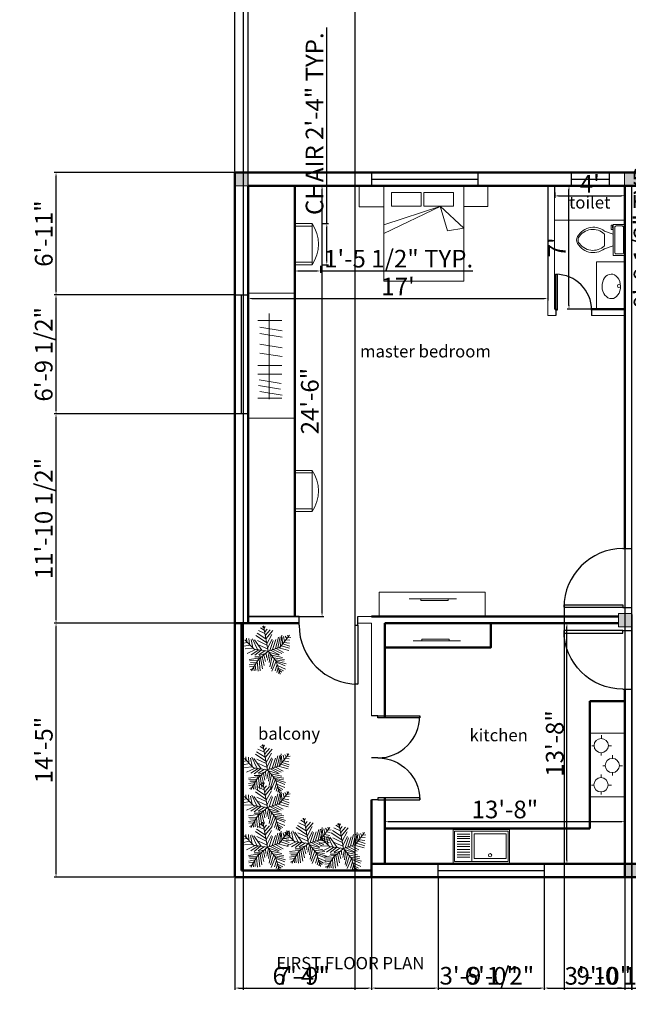
# Model space of a CAD drawing. Units: inches. Extents: x 1367 to 2309, y 1406 to 3826.
# Tile 4 of 9: x 1367 to 1781, y 2247 to 2918. Entities that reach past the tile are written whole.
import ezdxf

# ---------------------------------------------------------------- set-up
doc = ezdxf.new("R2010")
doc.units = ezdxf.units.IN
for name, color, linetype, lineweight in [('A-ANNO-DIMS', 2, 'Continuous', 18), ('A-ANNO-TEXT', 7, 'Continuous', 25), ('A-AREA-IDEN', 3, 'Continuous', 18), ('A-DOOR', 4, 'Continuous', 25), ('A-FLOR-FIXT', 8, 'Continuous', 18), ('A-FURN', 8, 'Continuous', 18), ('A-GLAZ', 4, 'Continuous', 25), ('A-WALL', 7, 'Continuous', 50), ('A-WALL-PATT', 8, 'Continuous', 18), ('garden', 80, 'Continuous', 18)]:
    doc.layers.add(name, color=color, linetype=linetype, lineweight=lineweight)
doc.styles.get("Standard").update_dxf_attribs({"font": 'arial.ttf'})
doc.dimstyles.new('ISO-25', dxfattribs={"dimtxt": 12, "dimasz": 2.5, "dimexe": 1.25, "dimexo": 0.625, "dimtad": 1, "dimdec": 0, "dimlunit": 4, "dimtxsty": 'Standard', "dimcen": 2.5, "dimadec": 0, "dimazin": 0, "dimtfac": 1, "dimtdec": 0, "dimtmove": 0, "dimatfit": 3, "dimfxl": 1, "dimarcsym": 0})

# ---------------------------------------------------------------- blocks, each defined once
blk = doc.blocks.new('*U2')
for p, q in [((0, 0), (0, -6)), ((40, 0), (40, -6))]:
    blk.add_line(p, q)
blk.add_lwpolyline([(0, 0), (0, 40), (1.75, 40), (1.75, 0)], close=True)
blk.add_arc((0, 0), 40, 0, 90)
blk = doc.blocks.new('*U4')
for p, q in [((9.5, -6), (9.5, -2)), ((-10, -8.5), (-8, -8.5)), ((-10, -9.5), (-10, -8.5)), ((-7, -9.5), (-10, -9.5)), ((-8, -8.5), (-8, -8)), ((-7, -8), (-7, -9.5)), ((-4, -8), (-6, -14)), ((4, -8), (6, -14)), ((4, -14), (-4, -14))]:
    blk.add_line(p, q)
blk.add_lwpolyline([(10.5, -8), (10.5, 0), (-10.5, 0), (-10.5, -8)], close=True)
for points in [[(-9.5, -2), (-9.5, -6)], [(8.5, -1), (-8.5, -1)], [(-8.5, -7), (8.5, -7)]]:
    blk.add_lwpolyline(points)
for centre, radius, start, end in [((-8.62, -1.88), 0.884, 81.8699, 188.1301), ((-8.62, -6.12), 0.884, 171.8699, 278.1301), ((8.62, -1.88), 0.884, 351.8699, 98.1301), ((8.62, -6.12), 0.884, 261.8699, 8.1301), ((3.52, -21.58), 12.17, 141.46911, 247.97143), ((4.2, -21.82), 11.33, 136.36773, 238.94682), ((-3.52, -21.58), 12.17, 292.02843, 38.53071), ((-4.2, -21.82), 11.33, 301.05301, 43.63209), ((0, -27.88), 4, 245.73182, 294.26817), ((0, -29), 4, 254.86053, 285.13947)]:
    blk.add_arc(centre, radius, start, end)
blk = doc.blocks.new('*U6')
for p, q in [((-7.288, 39.707), (-21.778, 46.673)), ((-8.737, 47.138), (-17.069, 52.711)), ((-10.186, 53.64), (-13.084, 55.962)), ((0, 0), (-10.5, 57)), ((-9.099, 51.782), (-6.563, 55.962)), ((-7.65, 43.423), (-2.578, 49.46)), ((-5.839, 35.992), (4.667, 48.067)), ((-5.114, 27.632), (10.463, 46.673)), ((-31.5, 4.5), (-52.5, 25.5)), ((-48.585, 21.131), (-49.309, 29.026)), ((-43.513, 28.561), (-42.427, 15.558)), ((-38.442, 26.239), (-34.819, 7.663)), ((-35.544, 28.097), (-24.314, 3.947)), ((-14.533, 2.09), (-30.834, 25.31)), ((-3.665, 19.273), (-27.574, 35.527)), ((-5.114, 28.097), (-24.676, 40.636)), ((-24.314, 23.917), (-2.941, 13.7)), ((-2.941, 16.486), (8.652, 37.85)), ((-1.129, 6.734), (9.014, 26.704)), ((3.942, 1.625), (11.187, 24.381)), ((10.101, 3.483), (17.708, 26.239)), ((16.259, 5.805), (23.142, 31.348)), ((22.055, 7.198), (27.489, 32.277)), ((27, 9), (48, 36)), ((27.127, 9.056), (31.112, 35.992)), ((31.836, 30.883), (32.561, 16.486)), ((35.096, 32.741), (37.27, 22.524)), ((38.719, 34.134), (41.979, 28.561)), ((40.53, 25.775), (48.862, 24.846)), ((43.791, 29.954), (51.036, 30.883)), ((44.153, 36.456), (45.239, 32.741)), ((-47.498, 19.737), (-55.83, 18.344)), ((-40.615, 13.7), (-55.105, 10.913)), ((-33.37, 6.269), (-52.207, 5.34)), ((-28.299, 3.483), (-47.86, -5.805)), ((-21.416, 3.018), (-38.079, -8.128)), ((0, 0), (-31.5, 4.5)), ((-15.982, 2.09), (-30.11, -9.521)), ((0, 0), (-22.5, -19.5)), ((-6.563, 1.161), (-21.416, -8.128)), ((-20.691, 13.7), (-1.129, 4.876)), ((0, 0), (27, 9)), ((0, 0), (18, -22.5)), ((6.478, 1.625), (26.04, -8.592)), ((11.187, 3.483), (30.749, -5.805)), ((18.07, 5.805), (35.096, -3.483)), ((24.229, 7.663), (46.688, 1.625)), ((29.662, 12.307), (48.137, 6.269)), ((33.285, 16.486), (48.862, 10.913)), ((36.183, 19.737), (48.137, 17.88)), ((-17.431, -15.094), (-42.789, -18.809)), ((-24.314, -21.596), (-42.427, -22.06)), ((-22.5, -19.5), (-37.5, -45)), ((-15.257, -12.772), (-30.11, -12.772)), ((-20.691, -18.345), (-17.793, -44.352)), ((-6.563, -5.805), (-19.967, -9.985)), ((-17.069, -15.094), (-12.721, -40.172)), ((-13.446, -11.378), (-8.737, -32.741)), ((-9.461, -8.592), (-6.201, -23.453)), ((-4.752, -3.483), (-3.665, -14.629)), ((2.493, -3.019), (-1.491, -20.202)), ((1.769, -2.555), (24.229, -9.521)), ((5.029, -6.27), (2.131, -25.775)), ((9.014, -11.378), (3.58, -35.992)), ((14.085, -16.951), (6.478, -40.172)), ((7.565, -9.056), (32.198, -14.629)), ((12.274, -15.094), (36.907, -18.809)), ((16.259, -19.738), (36.183, -22.989)), ((-28.299, -29.026), (-42.789, -31.348)), ((-30.834, -34.135), (-42.427, -35.528)), ((-34.457, -39.708), (-40.978, -42.494)), ((-26.849, -26.24), (-40.253, -25.775)), ((-32.646, -36.921), (-31.921, -44.352)), ((-29.023, -30.884), (-27.936, -43.887)), ((-25.038, -23.918), (-22.865, -45.281)), ((18.07, -22.524), (8.289, -45.745)), ((20.244, -30.419), (15.897, -44.816)), ((18, -22.5), (27, -52.5)), ((18.433, -22.524), (40.53, -29.026)), ((19.157, -25.311), (38.719, -33.206)), ((22.78, -37.85), (19.519, -48.532)), ((21.331, -32.741), (39.081, -40.636)), ((22.78, -38.314), (34.372, -44.816)), ((24.591, -43.423), (30.749, -47.603)), ((24.591, -45.745), (23.142, -50.854)), ((26.764, -49.925), (28.213, -50.854))]:
    blk.add_line(p, q)
blk = doc.blocks.new('*D7')
at = {"layer": 'A-ANNO-DIMS', "color": 0, "lineweight": -2, "transparency": 16777216}
for p, q in [((1522.37, 2804.54), (1522.37, 2727.05)), ((1726.37, 2804.54), (1726.37, 2727.05)), ((1524.87, 2728.3), (1723.87, 2728.3))]:
    blk.add_line(p, q, dxfattribs=at)
at = {"layer": 'A-ANNO-DIMS', "color": 0, "lineweight": 100, "transparency": 16777216}
for points in [[(1524.87, 2728.72), (1524.87, 2727.88), (1522.37, 2728.3)], [(1723.87, 2728.72), (1723.87, 2727.88), (1726.37, 2728.3)]]:
    blk.add_solid(points, dxfattribs=at)
at = {"layer": 'Defpoints', "color": 0, "lineweight": 100, "transparency": 16777216}
for p in [(1522.37, 2805.17), (1726.37, 2805.17), (1726.37, 2728.3)]:
    blk.add_point(p, dxfattribs=at)
at = {"layer": 'A-ANNO-DIMS', "color": 0, "transparency": 16777216, "insert": (1624.37, 2734.95), "char_height": 12, "attachment_point": 5}
blk.add_mtext("17'", dxfattribs=at)
blk = doc.blocks.new('*D8')
at = {"layer": 'A-ANNO-DIMS', "color": 0, "lineweight": -2, "transparency": 16777216}
for p, q in [((1523, 2805.17), (1573.89, 2805.17)), ((1572.64, 2514.16), (1572.64, 2802.67)), ((1523, 2511.66), (1573.89, 2511.66))]:
    blk.add_line(p, q, dxfattribs=at)
at = {"layer": 'A-ANNO-DIMS', "color": 0, "lineweight": 100, "transparency": 16777216}
for points in [[(1572.22, 2802.67), (1573.05, 2802.67), (1572.64, 2805.17)], [(1572.22, 2514.16), (1573.05, 2514.16), (1572.64, 2511.66)]]:
    blk.add_solid(points, dxfattribs=at)
at = {"layer": 'Defpoints', "color": 0, "lineweight": 100, "transparency": 16777216}
for p in [(1522.37, 2805.17), (1572.64, 2805.17), (1522.37, 2511.66)]:
    blk.add_point(p, dxfattribs=at)
at = {"layer": 'A-ANNO-DIMS', "color": 0, "transparency": 16777216, "insert": (1565.88, 2658.41), "char_height": 12, "attachment_point": 5, "rotation": 90}
blk.add_mtext('24\'-6"', dxfattribs=at)
blk = doc.blocks.new('*D9')
at = {"layer": 'A-ANNO-DIMS', "color": 0, "lineweight": -2, "transparency": 16777216}
for p, q in [((1730.99, 2804.4), (1731.01, 2796.99)), ((1778.87, 2804.54), (1778.89, 2797.12)), ((1733.51, 2798.24), (1776.39, 2798.37))]:
    blk.add_line(p, q, dxfattribs=at)
at = {"layer": 'A-ANNO-DIMS', "color": 0, "lineweight": 100, "transparency": 16777216}
for points in [[(1733.51, 2798.66), (1733.51, 2797.83), (1731.01, 2798.24)], [(1776.39, 2798.78), (1776.39, 2797.95), (1778.89, 2798.37)]]:
    blk.add_solid(points, dxfattribs=at)
at = {"layer": 'Defpoints', "color": 0, "lineweight": 100, "transparency": 16777216}
for p in [(1730.99, 2805.03), (1778.87, 2805.17), (1778.89, 2798.37)]:
    blk.add_point(p, dxfattribs=at)
at = {"layer": 'A-ANNO-DIMS', "color": 0, "transparency": 16777216, "insert": (1754.93, 2804.93), "char_height": 12, "attachment_point": 5, "rotation": 0.16425}
blk.add_mtext("4'", dxfattribs=at)
blk = doc.blocks.new('*D10')
at = {"layer": 'A-ANNO-DIMS', "color": 0, "lineweight": -2, "transparency": 16777216}
for p, q in [((1778.25, 2805.17), (1739.51, 2805.17)), ((1740.76, 2723.67), (1740.76, 2802.67)), ((1778.25, 2721.17), (1739.51, 2721.17))]:
    blk.add_line(p, q, dxfattribs=at)
at = {"layer": 'A-ANNO-DIMS', "color": 0, "lineweight": 100, "transparency": 16777216}
for points in [[(1740.35, 2802.67), (1741.18, 2802.67), (1740.76, 2805.17)], [(1740.35, 2723.67), (1741.18, 2723.67), (1740.76, 2721.17)]]:
    blk.add_solid(points, dxfattribs=at)
at = {"layer": 'Defpoints', "color": 0, "lineweight": 100, "transparency": 16777216}
for p in [(1740.76, 2805.17), (1778.87, 2805.17), (1778.87, 2721.17)]:
    blk.add_point(p, dxfattribs=at)
at = {"layer": 'A-ANNO-DIMS', "color": 0, "transparency": 16777216, "insert": (1734.14, 2763.17), "char_height": 12, "attachment_point": 5, "rotation": 90}
blk.add_mtext("7'", dxfattribs=at)
blk = doc.blocks.new('*D21')
at = {"layer": 'A-ANNO-DIMS', "color": 0, "lineweight": -2, "transparency": 16777216}
for p, q in [((1616, 2507.16), (1740.61, 2507.16)), ((1739.36, 2345.67), (1739.36, 2504.66)), ((1616, 2343.17), (1740.61, 2343.17))]:
    blk.add_line(p, q, dxfattribs=at)
at = {"layer": 'A-ANNO-DIMS', "color": 0, "lineweight": 100, "transparency": 16777216}
for points in [[(1738.94, 2504.66), (1739.77, 2504.66), (1739.36, 2507.16)], [(1738.94, 2345.67), (1739.77, 2345.67), (1739.36, 2343.17)]]:
    blk.add_solid(points, dxfattribs=at)
at = {"layer": 'Defpoints', "color": 0, "lineweight": 100, "transparency": 16777216}
for p in [(1615.37, 2507.16), (1739.36, 2507.16), (1615.37, 2343.17)]:
    blk.add_point(p, dxfattribs=at)
at = {"layer": 'A-ANNO-DIMS', "color": 0, "transparency": 16777216, "insert": (1732.6, 2425.16), "char_height": 12, "attachment_point": 5, "rotation": 90}
blk.add_mtext('13\'-8"', dxfattribs=at)
blk = doc.blocks.new('*D22')
at = {"layer": 'A-ANNO-DIMS', "color": 0, "lineweight": -2, "transparency": 16777216}
for p, q in [((1615.37, 2343.79), (1615.37, 2373.13)), ((1776.37, 2371.88), (1617.87, 2371.88)), ((1778.87, 2343.79), (1778.87, 2373.13))]:
    blk.add_line(p, q, dxfattribs=at)
at = {"layer": 'A-ANNO-DIMS', "color": 0, "lineweight": 100, "transparency": 16777216}
for points in [[(1617.87, 2372.3), (1617.87, 2371.46), (1615.37, 2371.88)], [(1776.37, 2372.3), (1776.37, 2371.46), (1778.87, 2371.88)]]:
    blk.add_solid(points, dxfattribs=at)
at = {"layer": 'Defpoints', "color": 0, "lineweight": 100, "transparency": 16777216}
for p in [(1615.37, 2371.88), (1615.37, 2343.17), (1778.87, 2343.17)]:
    blk.add_point(p, dxfattribs=at)
at = {"layer": 'A-ANNO-DIMS', "color": 0, "transparency": 16777216, "insert": (1697.12, 2378.64), "char_height": 12, "attachment_point": 5}
blk.add_mtext('13\'-8"', dxfattribs=at)
blk = doc.blocks.new('CHAIR')
for p, q in [((0, 28.09), (11.92, 28.09)), ((11.92, 28.09), (11.92, 24.96)), ((0, 0), (11.92, 0)), ((11.92, 0), (11.92, 2.65))]:
    blk.add_line(p, q)
blk.add_arc((-8.81, 14.05), 25.04, 325.88696, 34.11304)
blk = doc.blocks.new('BURNER')
blk.add_line((9.74, 4.72), (11.92, 4.72))
blk.add_circle((4.87, 4.87), 4.87)
blk = doc.blocks.new('*D48')
at = {"layer": 'A-ANNO-DIMS', "color": 0, "lineweight": -2, "transparency": 16777216}
for p, q in [((1799.19, 2718.44), (1799.19, 2823.29)), ((1798.02, 2718.44), (1800.44, 2718.44)), ((1799.19, 2711.2), (1799.19, 2715.94)), ((1798.02, 2708.7), (1800.44, 2708.7))]:
    blk.add_line(p, q, dxfattribs=at)
at = {"layer": 'A-ANNO-DIMS', "color": 0, "lineweight": 100, "transparency": 16777216}
for points in [[(1798.77, 2715.94), (1799.6, 2715.94), (1799.19, 2718.44)], [(1798.77, 2711.2), (1799.6, 2711.2), (1799.19, 2708.7)]]:
    blk.add_solid(points, dxfattribs=at)
at = {"layer": 'Defpoints', "color": 0, "lineweight": 100, "transparency": 16777216}
for p in [(1797.4, 2718.44), (1799.19, 2718.44), (1797.4, 2708.7)]:
    blk.add_point(p, dxfattribs=at)
at = {"layer": 'A-ANNO-DIMS', "color": 0, "transparency": 16777216, "insert": (1792.36, 2772.12), "char_height": 12, "attachment_point": 5, "rotation": 90}
blk.add_mtext('0\'-9 1/2" TYP.', dxfattribs=at)
blk = doc.blocks.new('*D49')
at = {"layer": 'A-ANNO-DIMS', "color": 0, "lineweight": -2, "transparency": 16777216}
for p, q in [((1575.88, 2779.38), (1575.88, 2912.95)), ((1572.29, 2779.38), (1577.13, 2779.38)), ((1575.88, 2753.79), (1575.88, 2776.88)), ((1572.29, 2751.29), (1577.13, 2751.29))]:
    blk.add_line(p, q, dxfattribs=at)
at = {"layer": 'A-ANNO-DIMS', "color": 0, "lineweight": 100, "transparency": 16777216}
for points in [[(1575.46, 2776.88), (1576.29, 2776.88), (1575.88, 2779.38)], [(1575.46, 2753.79), (1576.29, 2753.79), (1575.88, 2751.29)]]:
    blk.add_solid(points, dxfattribs=at)
at = {"layer": 'Defpoints', "color": 0, "lineweight": 100, "transparency": 16777216}
for p in [(1571.66, 2779.38), (1575.88, 2779.38), (1571.66, 2751.29)]:
    blk.add_point(p, dxfattribs=at)
at = {"layer": 'A-ANNO-DIMS', "color": 0, "transparency": 16777216, "insert": (1569.05, 2847.42), "char_height": 12, "attachment_point": 5, "rotation": 90}
blk.add_mtext('CHAIR 2\'-4" TYP.', dxfattribs=at)
blk = doc.blocks.new('*D50')
at = {"layer": 'A-ANNO-DIMS', "color": 0, "lineweight": -2, "transparency": 16777216}
for p, q in [((1554, 2750.67), (1554, 2745.83)), ((1571.66, 2750.67), (1571.66, 2745.83)), ((1556.5, 2747.08), (1569.16, 2747.08)), ((1571.66, 2747.08), (1675.39, 2747.08))]:
    blk.add_line(p, q, dxfattribs=at)
at = {"layer": 'A-ANNO-DIMS', "color": 0, "lineweight": 100, "transparency": 16777216}
for points in [[(1556.5, 2747.5), (1556.5, 2746.66), (1554, 2747.08)], [(1569.16, 2747.5), (1569.16, 2746.66), (1571.66, 2747.08)]]:
    blk.add_solid(points, dxfattribs=at)
at = {"layer": 'Defpoints', "color": 0, "lineweight": 100, "transparency": 16777216}
for p in [(1554, 2751.29), (1571.66, 2751.29), (1571.66, 2747.08)]:
    blk.add_point(p, dxfattribs=at)
at = {"layer": 'A-ANNO-DIMS', "color": 0, "transparency": 16777216, "insert": (1624.78, 2753.91), "char_height": 12, "attachment_point": 5}
blk.add_mtext('1\'-5 1/2" TYP.', dxfattribs=at)
blk = doc.blocks.new('*D87')
at = {"layer": 'A-ANNO-DIMS', "color": 0, "lineweight": -2, "transparency": 16777216}
for p, q in [((1513.37, 2814.79), (1513.37, 3802.6)), ((1515.87, 3801.35), (2110.9, 3801.35)), ((2113.4, 2814.79), (2113.4, 3802.6))]:
    blk.add_line(p, q, dxfattribs=at)
at = {"layer": 'A-ANNO-DIMS', "color": 0, "lineweight": 100, "transparency": 16777216}
for points in [[(1515.87, 3801.77), (1515.87, 3800.93), (1513.37, 3801.35)], [(2110.9, 3801.77), (2110.9, 3800.93), (2113.4, 3801.35)]]:
    blk.add_solid(points, dxfattribs=at)
at = {"layer": 'Defpoints', "color": 0, "lineweight": 100, "transparency": 16777216}
for p in [(2113.4, 3801.35), (1513.37, 2814.17), (2113.4, 2814.17)]:
    blk.add_point(p, dxfattribs=at)
at = {"layer": 'A-ANNO-DIMS', "color": 0, "transparency": 16777216, "insert": (1813.39, 3808.1), "char_height": 12, "attachment_point": 5}
blk.add_mtext('50\'-0"', dxfattribs=at)
blk = doc.blocks.new('*D88')
at = {"layer": 'A-ANNO-DIMS', "color": 0, "lineweight": -2, "transparency": 16777216}
for p, q in [((1513.37, 2814.79), (1513.37, 3802.6)), ((1515.87, 3801.35), (1519.87, 3801.35)), ((1522.37, 2805.79), (1522.37, 3802.6)), ((1522.37, 3801.35), (1558.02, 3801.35))]:
    blk.add_line(p, q, dxfattribs=at)
at = {"layer": 'A-ANNO-DIMS', "color": 0, "lineweight": 100, "transparency": 16777216}
for points in [[(1515.87, 3801.77), (1515.87, 3800.93), (1513.37, 3801.35)], [(1519.87, 3801.77), (1519.87, 3800.93), (1522.37, 3801.35)]]:
    blk.add_solid(points, dxfattribs=at)
at = {"layer": 'Defpoints', "color": 0, "lineweight": 100, "transparency": 16777216}
for p in [(1522.37, 3801.35), (1513.37, 2814.17), (1522.37, 2805.17)]:
    blk.add_point(p, dxfattribs=at)
at = {"layer": 'A-ANNO-DIMS', "color": 0, "transparency": 16777216, "insert": (1541.44, 3808.1), "char_height": 12, "attachment_point": 5}
blk.add_mtext('0\'-9"', dxfattribs=at)
blk = doc.blocks.new('*D90')
at = {"layer": 'A-ANNO-DIMS', "color": 0, "lineweight": -2, "transparency": 16777216}
for p, q in [((1512.75, 2507.16), (1390.27, 2507.16)), ((1391.52, 2336.67), (1391.52, 2504.66)), ((1512.75, 2334.17), (1390.27, 2334.17))]:
    blk.add_line(p, q, dxfattribs=at)
at = {"layer": 'A-ANNO-DIMS', "color": 0, "lineweight": 100, "transparency": 16777216}
for points in [[(1391.1, 2504.66), (1391.94, 2504.66), (1391.52, 2507.16)], [(1391.1, 2336.67), (1391.94, 2336.67), (1391.52, 2334.17)]]:
    blk.add_solid(points, dxfattribs=at)
at = {"layer": 'Defpoints', "color": 0, "lineweight": 100, "transparency": 16777216}
for p in [(1391.52, 2507.16), (1513.37, 2507.16), (1513.37, 2334.17)]:
    blk.add_point(p, dxfattribs=at)
at = {"layer": 'A-ANNO-DIMS', "color": 0, "transparency": 16777216, "insert": (1384.77, 2420.66), "char_height": 12, "attachment_point": 5, "rotation": 90}
blk.add_mtext('14\'-5"', dxfattribs=at)
blk = doc.blocks.new('*D91')
at = {"layer": 'A-ANNO-DIMS', "color": 0, "lineweight": -2, "transparency": 16777216}
for p, q in [((1512.75, 2649.67), (1390.27, 2649.67)), ((1391.52, 2509.66), (1391.52, 2647.17)), ((1512.75, 2507.16), (1390.27, 2507.16))]:
    blk.add_line(p, q, dxfattribs=at)
at = {"layer": 'A-ANNO-DIMS', "color": 0, "lineweight": 100, "transparency": 16777216}
for points in [[(1391.1, 2647.17), (1391.94, 2647.17), (1391.52, 2649.67)], [(1391.1, 2509.66), (1391.94, 2509.66), (1391.52, 2507.16)]]:
    blk.add_solid(points, dxfattribs=at)
at = {"layer": 'Defpoints', "color": 0, "lineweight": 100, "transparency": 16777216}
for p in [(1391.52, 2649.67), (1513.37, 2649.67), (1513.37, 2507.16)]:
    blk.add_point(p, dxfattribs=at)
at = {"layer": 'A-ANNO-DIMS', "color": 0, "transparency": 16777216, "insert": (1384.69, 2578.41), "char_height": 12, "attachment_point": 5, "rotation": 90}
blk.add_mtext('11\'-10 1/2"', dxfattribs=at)
blk = doc.blocks.new('*D92')
at = {"layer": 'A-ANNO-DIMS', "color": 0, "lineweight": -2, "transparency": 16777216}
for p, q in [((1512.75, 2730.92), (1390.27, 2730.92)), ((1391.52, 2652.17), (1391.52, 2728.42)), ((1512.75, 2649.67), (1390.27, 2649.67))]:
    blk.add_line(p, q, dxfattribs=at)
at = {"layer": 'A-ANNO-DIMS', "color": 0, "lineweight": 100, "transparency": 16777216}
for points in [[(1391.1, 2728.42), (1391.94, 2728.42), (1391.52, 2730.92)], [(1391.1, 2652.17), (1391.94, 2652.17), (1391.52, 2649.67)]]:
    blk.add_solid(points, dxfattribs=at)
at = {"layer": 'Defpoints', "color": 0, "lineweight": 100, "transparency": 16777216}
for p in [(1391.52, 2730.92), (1513.37, 2730.92), (1513.37, 2649.67)]:
    blk.add_point(p, dxfattribs=at)
at = {"layer": 'A-ANNO-DIMS', "color": 0, "transparency": 16777216, "insert": (1384.69, 2690.3), "char_height": 12, "attachment_point": 5, "rotation": 90}
blk.add_mtext('6\'-9 1/2"', dxfattribs=at)
blk = doc.blocks.new('*D93')
at = {"layer": 'A-ANNO-DIMS', "color": 0, "lineweight": -2, "transparency": 16777216}
for p, q in [((1512.75, 2814.17), (1390.27, 2814.17)), ((1391.52, 2733.42), (1391.52, 2811.67)), ((1512.75, 2730.92), (1390.27, 2730.92))]:
    blk.add_line(p, q, dxfattribs=at)
at = {"layer": 'A-ANNO-DIMS', "color": 0, "lineweight": 100, "transparency": 16777216}
for points in [[(1391.1, 2811.67), (1391.94, 2811.67), (1391.52, 2814.17)], [(1391.1, 2733.42), (1391.94, 2733.42), (1391.52, 2730.92)]]:
    blk.add_solid(points, dxfattribs=at)
at = {"layer": 'Defpoints', "color": 0, "lineweight": 100, "transparency": 16777216}
for p in [(1391.52, 2814.17), (1513.37, 2814.17), (1513.37, 2730.92)]:
    blk.add_point(p, dxfattribs=at)
at = {"layer": 'A-ANNO-DIMS', "color": 0, "transparency": 16777216, "insert": (1384.77, 2772.54), "char_height": 12, "attachment_point": 5, "rotation": 90}
blk.add_mtext('6\'-11"', dxfattribs=at)
blk = doc.blocks.new('*D94')
at = {"layer": 'A-ANNO-DIMS', "color": 0, "lineweight": -2, "transparency": 16777216}
for p, q in [((1513.37, 2333.54), (1513.37, 2257.28)), ((1606.37, 2333.54), (1606.37, 2257.28)), ((1515.87, 2258.53), (1603.87, 2258.53))]:
    blk.add_line(p, q, dxfattribs=at)
at = {"layer": 'A-ANNO-DIMS', "color": 0, "lineweight": 100, "transparency": 16777216}
for points in [[(1515.87, 2258.94), (1515.87, 2258.11), (1513.37, 2258.53)], [(1603.87, 2258.94), (1603.87, 2258.11), (1606.37, 2258.53)]]:
    blk.add_solid(points, dxfattribs=at)
at = {"layer": 'Defpoints', "color": 0, "lineweight": 100, "transparency": 16777216}
for p in [(1513.37, 2334.17), (1606.37, 2334.17), (1606.37, 2258.53)]:
    blk.add_point(p, dxfattribs=at)
at = {"layer": 'A-ANNO-DIMS', "color": 0, "transparency": 16777216, "insert": (1559.87, 2265.28), "char_height": 12, "attachment_point": 5}
blk.add_mtext('7\'-9"', dxfattribs=at)
blk = doc.blocks.new('*D95')
at = {"layer": 'A-ANNO-DIMS', "color": 0, "lineweight": -2, "transparency": 16777216}
for p, q in [((1606.37, 2333.54), (1606.37, 2257.28)), ((1651.78, 2333.54), (1651.78, 2257.28)), ((1608.87, 2258.53), (1649.28, 2258.53)), ((1651.78, 2258.53), (1715.38, 2258.53))]:
    blk.add_line(p, q, dxfattribs=at)
at = {"layer": 'A-ANNO-DIMS', "color": 0, "lineweight": 100, "transparency": 16777216}
for points in [[(1608.87, 2258.94), (1608.87, 2258.11), (1606.37, 2258.53)], [(1649.28, 2258.94), (1649.28, 2258.11), (1651.78, 2258.53)]]:
    blk.add_solid(points, dxfattribs=at)
at = {"layer": 'Defpoints', "color": 0, "lineweight": 100, "transparency": 16777216}
for p in [(1606.37, 2334.17), (1651.78, 2334.17), (1651.78, 2258.53)]:
    blk.add_point(p, dxfattribs=at)
at = {"layer": 'A-ANNO-DIMS', "color": 0, "transparency": 16777216, "insert": (1684.83, 2265.36), "char_height": 12, "attachment_point": 5}
blk.add_mtext('3\'-9 1/2"', dxfattribs=at)
blk = doc.blocks.new('*D96')
at = {"layer": 'A-ANNO-DIMS', "color": 0, "lineweight": -2, "transparency": 16777216}
for p, q in [((1651.78, 2333.54), (1651.78, 2257.28)), ((1723.94, 2333.54), (1723.94, 2257.28)), ((1654.28, 2258.53), (1721.44, 2258.53))]:
    blk.add_line(p, q, dxfattribs=at)
at = {"layer": 'A-ANNO-DIMS', "color": 0, "lineweight": 100, "transparency": 16777216}
for points in [[(1654.28, 2258.94), (1654.28, 2258.11), (1651.78, 2258.53)], [(1721.44, 2258.94), (1721.44, 2258.11), (1723.94, 2258.53)]]:
    blk.add_solid(points, dxfattribs=at)
at = {"layer": 'Defpoints', "color": 0, "lineweight": 100, "transparency": 16777216}
for p in [(1651.78, 2334.17), (1723.94, 2334.17), (1723.94, 2258.53)]:
    blk.add_point(p, dxfattribs=at)
at = {"layer": 'A-ANNO-DIMS', "color": 0, "transparency": 16777216, "insert": (1687.86, 2265.28), "char_height": 12, "attachment_point": 5}
blk.add_mtext('6\'-0"', dxfattribs=at)
blk = doc.blocks.new('*D97')
at = {"layer": 'A-ANNO-DIMS', "color": 0, "lineweight": -2, "transparency": 16777216}
for p, q in [((1723.94, 2333.54), (1723.94, 2257.28)), ((1832.26, 2333.54), (1832.26, 2257.28)), ((1726.44, 2258.53), (1829.76, 2258.53))]:
    blk.add_line(p, q, dxfattribs=at)
at = {"layer": 'A-ANNO-DIMS', "color": 0, "lineweight": 100, "transparency": 16777216}
for points in [[(1726.44, 2258.94), (1726.44, 2258.11), (1723.94, 2258.53)], [(1829.76, 2258.94), (1829.76, 2258.11), (1832.26, 2258.53)]]:
    blk.add_solid(points, dxfattribs=at)
at = {"layer": 'Defpoints', "color": 0, "lineweight": 100, "transparency": 16777216}
for p in [(1723.94, 2334.17), (1832.26, 2334.17), (1832.26, 2258.53)]:
    blk.add_point(p, dxfattribs=at)
at = {"layer": 'A-ANNO-DIMS', "color": 0, "transparency": 16777216, "insert": (1778.1, 2265.35), "char_height": 12, "attachment_point": 5}
blk.add_mtext('9\'-0 1/2"', dxfattribs=at)
blk = doc.blocks.new('*D102')
at = {"layer": 'A-ANNO-DIMS', "color": 0, "lineweight": -2, "transparency": 16777216}
for p, q in [((1778.87, 2804.54), (1778.87, 2257.28)), ((1783.37, 2804.54), (1783.37, 2257.28)), ((1776.37, 2258.53), (1773.87, 2258.53)), ((1778.87, 2258.53), (1783.37, 2258.53)), ((1785.87, 2258.53), (1849.48, 2258.53))]:
    blk.add_line(p, q, dxfattribs=at)
at = {"layer": 'A-ANNO-DIMS', "color": 0, "lineweight": 100, "transparency": 16777216}
for points in [[(1776.37, 2258.94), (1776.37, 2258.11), (1778.87, 2258.53)], [(1785.87, 2258.94), (1785.87, 2258.11), (1783.37, 2258.53)]]:
    blk.add_solid(points, dxfattribs=at)
at = {"layer": 'Defpoints', "color": 0, "lineweight": 100, "transparency": 16777216}
for p in [(1778.87, 2805.17), (1783.37, 2805.17), (1783.37, 2258.53)]:
    blk.add_point(p, dxfattribs=at)
at = {"layer": 'A-ANNO-DIMS', "color": 0, "transparency": 16777216, "insert": (1818.93, 2265.35), "char_height": 12, "attachment_point": 5}
blk.add_mtext('0\'-4 1/2"', dxfattribs=at)
blk = doc.blocks.new('*D127')
at = {"layer": 'A-ANNO-DIMS', "color": 0, "lineweight": -2, "transparency": 16777216}
for p, q in [((1519.02, 3450.71), (1519.02, 2257.28)), ((1594.94, 3450.71), (1594.94, 2257.28)), ((1521.52, 2258.53), (1592.44, 2258.53))]:
    blk.add_line(p, q, dxfattribs=at)
at = {"layer": 'A-ANNO-DIMS', "color": 0, "lineweight": 100, "transparency": 16777216}
for points in [[(1521.52, 2258.94), (1521.52, 2258.11), (1519.02, 2258.53)], [(1592.44, 2258.94), (1592.44, 2258.11), (1594.94, 2258.53)]]:
    blk.add_solid(points, dxfattribs=at)
at = {"layer": 'Defpoints', "color": 0, "lineweight": 100, "transparency": 16777216}
for p in [(1519.02, 3451.33), (1594.94, 3451.33), (1594.94, 2258.53)]:
    blk.add_point(p, dxfattribs=at)
at = {"layer": 'A-ANNO-DIMS', "color": 0, "transparency": 16777216, "insert": (1556.98, 2265.28), "char_height": 12, "attachment_point": 5}
blk.add_mtext('6\'-4"', dxfattribs=at)
blk = doc.blocks.new('*D138')
at = {"layer": 'A-ANNO-DIMS', "color": 0, "lineweight": -2, "transparency": 16777216}
for p, q in [((1737.37, 2517.27), (1737.37, 2257.28)), ((1783.44, 2513.11), (1783.44, 2257.28)), ((1739.87, 2258.53), (1780.94, 2258.53))]:
    blk.add_line(p, q, dxfattribs=at)
at = {"layer": 'A-ANNO-DIMS', "color": 0, "lineweight": 100, "transparency": 16777216}
for points in [[(1739.87, 2258.94), (1739.87, 2258.11), (1737.37, 2258.53)], [(1780.94, 2258.94), (1780.94, 2258.11), (1783.44, 2258.53)]]:
    blk.add_solid(points, dxfattribs=at)
at = {"layer": 'Defpoints', "color": 0, "lineweight": 100, "transparency": 16777216}
for p in [(1737.37, 2517.89), (1783.44, 2513.73), (1783.44, 2258.53)]:
    blk.add_point(p, dxfattribs=at)
at = {"layer": 'A-ANNO-DIMS', "color": 0, "transparency": 16777216, "insert": (1760.4, 2265.28), "char_height": 12, "attachment_point": 5}
blk.add_mtext('3\'-10"', dxfattribs=at)

msp = doc.modelspace()

# ---------------------------------------------------------------- hatches: boundary and pattern name
at = {"layer": 'A-WALL-PATT'}
h = msp.add_hatch(color=256, dxfattribs=at)
h.dxf.hatch_style = 1
h.paths.add_polyline_path([(1513.37, 2983.62), (1504.37, 2983.62), (1504.37, 2974.62), (1513.37, 2974.62)])
h.paths.add_polyline_path([(1759.42, 2983.62), (1749.82, 2983.62), (1749.82, 2974.62), (1759.42, 2974.62)])
h.paths.add_polyline_path([(1513.37, 3283.62), (1504.37, 3283.62), (1504.37, 3274.62), (1513.37, 3274.62)])
h.paths.add_polyline_path([(1759.42, 3283.62), (1750.75, 3283.62), (1750.75, 3274.62), (1759.42, 3274.62)])
h.paths.add_polyline_path([(2113.4, 2983.62), (2104.4, 2983.62), (2104.4, 2974.62), (2113.4, 2974.62)])
h.paths.add_polyline_path([(1787.87, 2343.17), (1778.87, 2343.17), (1778.87, 2334.17), (1787.87, 2334.17)])
h.paths.add_polyline_path([(1964.87, 2343.17), (1960.37, 2343.17), (1955.87, 2343.17), (1955.87, 2334.17), (1964.87, 2334.17)])
h.paths.add_polyline_path([(2113.37, 2343.17), (2104.37, 2343.17), (2104.37, 2334.17), (2113.37, 2334.17)])
h.paths.add_polyline_path([(1783.37, 2513.73), (1774.44, 2513.73), (1774.44, 2504.73), (1783.37, 2504.73)])
h.paths.add_polyline_path([(1787.54, 2814.17), (1778.54, 2814.17), (1778.54, 2805.17), (1787.54, 2805.17)])
h.paths.add_polyline_path([(1964.87, 2814.17), (1955.87, 2814.17), (1955.87, 2805.17), (1964.87, 2805.17)])
h.paths.add_polyline_path([(2113.37, 2814.17), (2104.4, 2814.17), (2104.4, 2805.17), (2113.37, 2805.17)])
h.paths.add_polyline_path([(1522.37, 2814.17), (1513.37, 2814.17), (1513.37, 2805.17), (1522.37, 2805.17)])
h.paths.add_polyline_path([(2019.97, 2440.35), (2070.2, 2440.35), (2070.2, 2457.56), (2019.97, 2457.56)], flags=9)
h.paths.add_polyline_path([(1670.17, 2422.1), (1711.32, 2422.1), (1711.32, 2439.31), (1670.17, 2439.31)], flags=9)
h.paths.add_polyline_path([(1917.64, 2783.38), (1946.46, 2783.38), (1946.46, 2800.59), (1917.64, 2800.59)], flags=9)
h.paths.add_polyline_path([(1526.17, 2423.16), (1570.57, 2423.16), (1570.57, 2440.37), (1526.17, 2440.37)], flags=9)
h.paths.add_polyline_path([(2013.98, 2676.57), (2064.21, 2676.57), (2064.21, 2693.79), (2013.98, 2693.79)], flags=9)
h.paths.add_polyline_path([(1738.47, 2785.04), (1767.29, 2785.04), (1767.29, 2802.25), (1738.47, 2802.25)], flags=9)
h.paths.add_polyline_path([(1832.32, 2473.89), (1889.69, 2473.89), (1889.69, 2491.1), (1832.32, 2491.1)], flags=9)
h.paths.add_polyline_path([(1821.9, 2712.75), (1863.05, 2712.75), (1863.05, 2729.96), (1821.9, 2729.96)], flags=9)
h.paths.add_polyline_path([(1595.64, 2683.62), (1684.77, 2683.62), (1684.77, 2700.83), (1595.64, 2700.83)], flags=9)

# ---------------------------------------------------------------- linework, layer by layer
at = {"layer": 'A-FURN'}
for p, q in [((1726.37, 2716.67), (1726.37, 2805.17)), ((1730.87, 2721.17), (1730.87, 2805.17)), ((1653.47, 2791.33), (1614.65, 2778.61)), ((1653.47, 2791.33), (1614.65, 2772.7)), ((1653.13, 2791.17), (1669.21, 2776.31)), ((1657.99, 2774.36), (1653.13, 2791.17)), ((1778.87, 2781.67), (1730.87, 2781.67)), ((1669.21, 2776.31), (1657.99, 2774.36)), ((1536.66, 2659.64), (1536.66, 2718.16)), ((1732.77, 2721.17), (1730.87, 2721.17)), ((1529.01, 2713.35), (1545.27, 2713.35)), ((1731.69, 2716.67), (1726.37, 2716.67)), ((1778.87, 2716.67), (1756.18, 2716.67)), ((1530.33, 2708.72), (1545.42, 2706.26)), ((1530.33, 2704.38), (1545.42, 2701.93)), ((1530.33, 2697.23), (1545.42, 2694.77)), ((1530.33, 2691.16), (1545.42, 2688.7)), ((1529.01, 2682.79), (1545.27, 2682.79)), ((1529.01, 2676.72), (1545.27, 2676.72)), ((1529.76, 2672.86), (1544.86, 2670.4)), ((1529.34, 2668.96), (1544.43, 2666.5)), ((1530.33, 2664.88), (1545.42, 2662.42)), ((1529.01, 2660.53), (1545.27, 2660.53)), ((1664.26, 2523.72), (1632.01, 2523.72)), ((1778.87, 2517.89), (1778.87, 2513.73)), ((1610.87, 2511.66), (1596.99, 2511.66)), ((1606.37, 2507.16), (1596.99, 2507.16)), ((1606.37, 2443.91), (1606.37, 2507.16)), ((1778.87, 2504.73), (1778.87, 2502.15)), ((1634.74, 2495.1), (1667, 2495.1)), ((1762.92, 2428.58), (1762.92, 2430.72)), ((1757.82, 2423.56), (1756.25, 2423.56)), ((1615.37, 2414.97), (1615.37, 2415.75)), ((1762.75, 2418.84), (1762.75, 2416.97)), ((1770.45, 2415.02), (1770.45, 2417.17)), ((1765.35, 2410.01), (1763.77, 2410.01)), ((1762.77, 2401.89), (1762.77, 2404.03)), ((1770.27, 2405.29), (1770.27, 2403.42)), ((1757.67, 2396.87), (1756.1, 2396.87)), ((1762.6, 2392.15), (1762.6, 2390.29)), ((1673.33, 2363.47), (1664.73, 2363.47)), ((1673.33, 2361.78), (1664.73, 2361.78)), ((1674.62, 2365.53), (1674.62, 2344.7)), ((1673.33, 2360.32), (1664.73, 2360.32)), ((1673.33, 2358.47), (1664.73, 2358.47)), ((1673.33, 2356.61), (1664.73, 2356.61)), ((1673.33, 2354.87), (1664.73, 2354.87)), ((1673.33, 2353.01), (1664.73, 2353.01)), ((1673.33, 2351.05), (1664.73, 2351.05)), ((1673.33, 2349.36), (1664.73, 2349.36)), ((1673.33, 2347.72), (1664.73, 2347.72))]:
    msp.add_line(p, q, dxfattribs=at)
for points in [[(1513.37, 2814.17), (1522.37, 2814.17), (1522.37, 2805.17), (1513.37, 2805.17)], [(1778.54, 2814.17), (1787.54, 2814.17), (1787.54, 2805.17), (1778.54, 2805.17)], [(1614.65, 2805.17), (1597.83, 2805.17), (1597.83, 2790.76), (1614.65, 2790.76)], [(1614.65, 2805.17), (1669.21, 2805.17), (1669.21, 2740.23), (1614.65, 2740.23)], [(1669.21, 2805.17), (1685.48, 2805.17), (1685.48, 2790.9), (1669.21, 2790.9)], [(1620.02, 2800.54), (1640.21, 2800.54), (1640.21, 2791.33), (1620.02, 2791.33)], [(1641.89, 2800.54), (1662.08, 2800.54), (1662.08, 2791.33), (1641.89, 2791.33)], [(1554, 2777.69), (1565.92, 2777.69), (1565.92, 2753.17), (1554, 2753.17)], [(1759.52, 2721.17), (1778.87, 2721.17), (1778.87, 2753.34), (1759.52, 2753.34)], [(1554, 2646.77), (1522.37, 2646.77), (1522.37, 2732.03), (1554, 2732.03)], [(1554, 2609.56), (1565.92, 2609.56), (1565.92, 2585.04), (1554, 2585.04)], [(1683.64, 2511.66), (1611.46, 2511.66), (1611.46, 2528.26), (1683.64, 2528.26)], [(1658.41, 2523.72), (1639.83, 2523.72), (1639.83, 2522.5), (1658.41, 2522.5)], [(1774.44, 2513.73), (1783.44, 2513.73), (1783.44, 2504.73), (1774.44, 2504.73)], [(1640.59, 2495.1), (1659.17, 2495.1), (1659.17, 2496.32), (1640.59, 2496.32)], [(1754.87, 2388.92), (1778.61, 2388.91), (1778.61, 2432.29), (1754.87, 2432.3)], [(1700.34, 2366.53), (1661.83, 2366.53), (1661.83, 2343.7), (1700.34, 2343.7)], [(1699.34, 2365.53), (1662.83, 2365.53), (1662.83, 2344.7), (1699.34, 2344.7)], [(1697.91, 2346.78), (1676.15, 2346.78), (1676.15, 2363.69), (1697.91, 2363.69)]]:
    msp.add_lwpolyline(points, close=True, dxfattribs=at)
for centre, radius in [((1774.77, 2736.86), 1.06), ((1687.06, 2349.03), 1.12)]:
    msp.add_circle(centre, radius, dxfattribs=at)
msp.add_ellipse((1769.56, 2736.6), major_axis=(-0.17, 8.38), ratio=0.747916, dxfattribs=at)
at = {"layer": 'A-GLAZ'}
for p, q in [((1606.52, 2809.67), (1678.68, 2809.67)), ((1704.76, 2805.17), (1656.76, 2805.17)), ((1742.34, 2809.67), (1768.4, 2809.67)), ((1517.87, 2649.67), (1517.87, 2730.92)), ((1556.99, 2511.66), (1522.37, 2511.66)), ((1651.78, 2338.67), (1723.94, 2338.67))]:
    msp.add_line(p, q, dxfattribs=at)
for points in [[(1606.52, 2814.17), (1678.68, 2814.17), (1678.68, 2805.17), (1606.52, 2805.17)], [(1742.34, 2805.17), (1768.4, 2805.17), (1768.4, 2814.17), (1742.34, 2814.17)], [(1513.37, 2730.92), (1522.37, 2730.92), (1522.37, 2649.67), (1513.37, 2649.67)], [(1651.78, 2343.17), (1723.94, 2343.17), (1723.94, 2334.17), (1651.78, 2334.17)]]:
    msp.add_lwpolyline(points, close=True, dxfattribs=at)
at = {"layer": 'A-WALL'}
for p, q in [((1522.37, 2805.17), (1751.02, 2805.17)), ((1554, 2511.66), (1554, 2805.17)), ((1778.87, 2596.67), (1778.87, 2805.17)), ((1778.87, 2805.17), (1778.87, 2721.17)), ((1778.87, 2721.17), (1756.17, 2721.17)), ((1778.87, 2596.67), (1778.87, 2557.89)), ((1774.44, 2511.66), (1606.37, 2511.66)), ((1522.37, 2507.16), (1513.37, 2507.16)), ((1517.87, 2507.16), (1517.87, 2338.67)), ((1556.99, 2507.16), (1522.37, 2507.16)), ((1615.37, 2442.66), (1615.37, 2507.16)), ((1774.44, 2507.16), (1615.37, 2507.16)), ((1778.87, 2462.15), (1778.87, 2343.17)), ((1778.87, 2454.05), (1754.87, 2454.05)), ((1754.87, 2454.05), (1754.87, 2367.17)), ((1606.37, 2343.17), (1606.37, 2386.81)), ((1615.37, 2343.17), (1615.37, 2388.06)), ((1615.37, 2343.17), (1615.37, 2367.17)), ((1615.37, 2367.17), (1754.87, 2367.17)), ((1658.87, 2343.17), (1606.37, 2343.17)), ((1606.37, 2343.17), (1610.87, 2343.17)), ((1606.37, 2343.17), (1606.37, 2334.17)), ((1778.87, 2343.17), (1658.87, 2343.17)), ((1606.37, 2338.67), (1517.87, 2338.67))]:
    msp.add_line(p, q, dxfattribs=at)
for points in [[(1513.37, 2334.17), (2113.37, 2334.17), (2113.37, 2814.17), (1513.37, 2814.17)], [(1615.37, 2507.16), (1687.55, 2507.16), (1687.55, 2490.56), (1615.37, 2490.56)], [(1778.87, 2343.17), (1787.87, 2343.17), (1787.87, 2334.17), (1778.87, 2334.17)]]:
    msp.add_lwpolyline(points, close=True, dxfattribs=at)
for points in [[(2104.37, 2511.66), (2104.37, 2805.17), (1522.37, 2805.17), (1522.37, 2507.16)], [(1606.37, 2343.17), (1955.87, 2343.17)]]:
    msp.add_lwpolyline(points, dxfattribs=at)

# ---------------------------------------------------------------- block references
at = {"layer": 'A-DOOR', "xscale": 0.6122238826041507, "yscale": 0.6122238826041507, "zscale": 0.6122238826041507}
msp.add_blockref('*U2', (1731.69, 2720.34), dxfattribs=at)
at = {"layer": 'A-DOOR'}
for p, rotation in [((1777.37, 2517.89), 90), ((1596.99, 2505.66), 180)]:
    msp.add_blockref('*U2', p, dxfattribs=dict(at, rotation=rotation))
at = {"layer": 'A-DOOR', "xscale": -1, "rotation": 90}
msp.add_blockref('*U2', (1777.37, 2502.15), dxfattribs=at)
at = {"layer": 'A-DOOR', "yscale": 0.7137788175399543, "zscale": 0.7137788175399543, "rotation": 270}
for p, xscale in [((1610.65, 2443.91), 0.7137788175399543), ((1610.65, 2386.81), -0.7137788175399543)]:
    msp.add_blockref('*U2', p, dxfattribs=dict(at, xscale=xscale))
at = {"layer": 'A-FLOR-FIXT', "rotation": 270}
msp.add_blockref('*U4', (1778.87, 2768.23), dxfattribs=at)
at = {"layer": 'A-FLOR-FIXT'}
for p in [(1757.82, 2418.84), (1765.35, 2405.29), (1757.67, 2392.15)]:
    msp.add_blockref('BURNER', p, dxfattribs=at)
at = {"layer": 'A-FURN'}
for p in [(1554, 2751.29), (1554, 2583.16)]:
    msp.add_blockref('CHAIR', p, dxfattribs=at)
at = {"layer": 'garden', "xscale": 0.3008057426392026, "yscale": 0.3008057426392026, "zscale": 0.3008057426392026}
for p in [(1535.94, 2488.1), (1535.54, 2407.29), (1535.54, 2381.48), (1535.54, 2354.52), (1563.39, 2357.13), (1587.19, 2353.65)]:
    msp.add_blockref('*U6', p, dxfattribs=at)

# ---------------------------------------------------------------- texts
at = {"layer": 'A-ANNO-TEXT', "insert": (1541.53, 2279.69), "char_height": 8.3529, "attachment_point": 1}
msp.add_mtext_dynamic_manual_height_columns('FIRST FLOOR PLAN', width=204.251, gutter_width=41.76, heights=[0], dxfattribs=at)
at = {"layer": 'A-AREA-IDEN', "attachment_point": 1}
for s, insert, char_height in [('toilet', (1740.76, 2797.95), 8.353), ('master bedroom', (1598.49, 2696.53), 8.3529), ('balcony', (1529.02, 2436.07), 8.353), ('kitchen', (1673.03, 2435.01), 8.353)]:
    msp.add_mtext_dynamic_manual_height_columns(s, width=204.251, gutter_width=41.76, heights=[0], dxfattribs=dict(at, insert=insert, char_height=char_height))

# ---------------------------------------------------------------- dimensions: what is measured, and where the dimension line sits
at = {"layer": 'A-ANNO-DIMS'}
for base, p1, p2, override, picture, middle in [((2113.4, 3801.35), (1513.37, 2814.17), (2113.4, 2814.17), {"dimdec": 1, "dimlfac": 1, "dimrnd": 0, "dimzin": 1, "dimdsep": 46, "dimlunit": 4, "dimfrac": 2}, '*D87', (1813.39, 3808.1)), ((1522.37, 3801.35), (1513.37, 2814.17), (1522.37, 2805.17), {"dimdec": 1, "dimlfac": 1, "dimrnd": 0, "dimzin": 1, "dimdsep": 46, "dimlunit": 4, "dimfrac": 2}, '*D88', (1541.44, 3808.1)), ((1594.94, 2258.53), (1519.02, 3451.33), (1594.94, 3451.33), {"dimdec": 1, "dimlfac": 1, "dimrnd": 0, "dimzin": 1, "dimdsep": 46, "dimlunit": 4, "dimfrac": 2}, '*D127', (1556.98, 2265.28)), ((1726.37, 2728.3), (1522.37, 2805.17), (1726.37, 2805.17), {"dimclrd": 0, "dimclre": 0, "dimclrt": 0}, '*D7', (1624.37, 2734.95)), ((1783.37, 2258.53), (1778.87, 2805.17), (1783.37, 2805.17), {"dimdec": 1, "dimlfac": 1, "dimrnd": 0, "dimzin": 1, "dimdsep": 46, "dimlunit": 4, "dimfrac": 2}, '*D102', (1818.93, 2265.35)), ((1783.44, 2258.53), (1737.37, 2517.89), (1783.44, 2513.73), {"dimdec": 1, "dimlfac": 1, "dimrnd": 0, "dimzin": 1, "dimdsep": 46, "dimlunit": 4, "dimfrac": 2}, '*D138', (1760.4, 2265.28)), ((1615.37014092, 2371.87986946), (1778.87014092, 2343.1663303), (1615.37014092, 2343.1663303), {"dimclrd": 0, "dimclre": 0, "dimclrt": 0}, '*D22', (1697.12014092, 2378.63583808)), ((1606.37, 2258.53), (1513.37, 2334.17), (1606.37, 2334.17), {"dimdec": 1, "dimlfac": 1, "dimrnd": 0, "dimzin": 1, "dimdsep": 46, "dimlunit": 4, "dimfrac": 2}, '*D94', (1559.87, 2265.28)), ((1651.78, 2258.53), (1606.37, 2334.17), (1651.78, 2334.17), {"dimdec": 1, "dimlfac": 1, "dimrnd": 0, "dimzin": 1, "dimdsep": 46, "dimlunit": 4, "dimfrac": 2}, '*D95', (1684.83, 2265.36)), ((1723.94, 2258.53), (1651.78, 2334.17), (1723.94, 2334.17), {"dimdec": 1, "dimlfac": 1, "dimrnd": 0, "dimzin": 1, "dimdsep": 46, "dimlunit": 4, "dimfrac": 2}, '*D96', (1687.86, 2265.28)), ((1832.26, 2258.53), (1723.94, 2334.17), (1832.26, 2334.17), {"dimdec": 1, "dimlfac": 1, "dimrnd": 0, "dimzin": 1, "dimdsep": 46, "dimlunit": 4, "dimfrac": 2}, '*D97', (1778.1, 2265.35))]:
    dim = msp.add_linear_dim(base=base, p1=p1, p2=p2, dimstyle='ISO-25', override=override, dxfattribs=at)
    dim.commit()
    dim.dimension.update_dxf_attribs({"geometry": picture, "text_midpoint": middle})
for base, p1, p2, text, picture, middle in [((1575.88, 2779.38), (1571.66, 2751.29), (1571.66, 2779.38), 'CHAIR <> TYP.', '*D49', (1569.05, 2847.42)), ((1799.19, 2718.44), (1797.4, 2708.7), (1797.4, 2718.44), '<> TYP.', '*D48', (1792.36, 2772.12))]:
    dim = msp.add_linear_dim(base=base, p1=p1, p2=p2, angle=90, text=text, dimstyle='ISO-25', override={"dimdec": 1, "dimrnd": 0, "dimzin": 1, "dimlunit": 4, "dimfrac": 2}, dxfattribs=at)
    dim.commit()
    dim.dimension.update_dxf_attribs({"geometry": picture, "text_midpoint": middle})
for base, p1, p2, override, picture, middle in [((1391.5196, 2814.1663), (1513.3701, 2730.9224), (1513.3701, 2814.1663), {"dimdec": 1, "dimlfac": 1, "dimrnd": 0, "dimzin": 1, "dimdsep": 46, "dimlunit": 4, "dimfrac": 2}, '*D93', (1384.7677, 2772.5444)), ((1572.64, 2805.17), (1522.37, 2511.66), (1522.37, 2805.17), {"dimclrd": 0, "dimclre": 0, "dimclrt": 0}, '*D8', (1565.88, 2658.41)), ((1740.76, 2805.17), (1778.87, 2721.17), (1778.87, 2805.17), {"dimclrd": 0, "dimclre": 0, "dimclrt": 0}, '*D10', (1734.14, 2763.17)), ((1391.5196, 2730.9224), (1513.3701, 2649.6703), (1513.3701, 2730.9224), {"dimdec": 1, "dimlfac": 1, "dimrnd": 0, "dimzin": 1, "dimdsep": 46, "dimlunit": 4, "dimfrac": 2}, '*D92', (1384.69, 2690.2964)), ((1391.52, 2649.67), (1513.37, 2507.16), (1513.37, 2649.67), {"dimdec": 1, "dimlfac": 1, "dimrnd": 0, "dimzin": 1, "dimdsep": 46, "dimlunit": 4, "dimfrac": 2}, '*D91', (1384.69, 2578.41)), ((1391.52, 2507.16), (1513.37, 2334.17), (1513.37, 2507.16), {"dimdec": 1, "dimlfac": 1, "dimrnd": 0, "dimzin": 1, "dimdsep": 46, "dimlunit": 4, "dimfrac": 2}, '*D90', (1384.77, 2420.66)), ((1739.36, 2507.16), (1615.37, 2343.17), (1615.37, 2507.16), {"dimclrd": 0, "dimclre": 0, "dimclrt": 0}, '*D21', (1732.6, 2425.16))]:
    dim = msp.add_linear_dim(base=base, p1=p1, p2=p2, angle=90, dimstyle='ISO-25', override=override, dxfattribs=at)
    dim.commit()
    dim.dimension.update_dxf_attribs({"geometry": picture, "text_midpoint": middle})
dim = msp.add_aligned_dim(p1=(1730.99, 2805.03), p2=(1778.87, 2805.17), distance=-6.79, dimstyle='ISO-25', override={"dimclrd": 0, "dimclre": 0, "dimclrt": 0}, dxfattribs=at)
dim.commit()
dim.dimension.update_dxf_attribs({"geometry": '*D9', "text_midpoint": (1754.93, 2804.93)})
dim = msp.add_linear_dim(base=(1571.66, 2747.08), p1=(1554, 2751.29), p2=(1571.66, 2751.29), text='<> TYP.', dimstyle='ISO-25', override={"dimdec": 1, "dimrnd": 0, "dimzin": 1, "dimlunit": 4, "dimfrac": 2}, dxfattribs=at)
dim.commit()
dim.dimension.update_dxf_attribs({"geometry": '*D50', "text_midpoint": (1624.78, 2753.91)})

doc.saveas('drawing.dxf')
